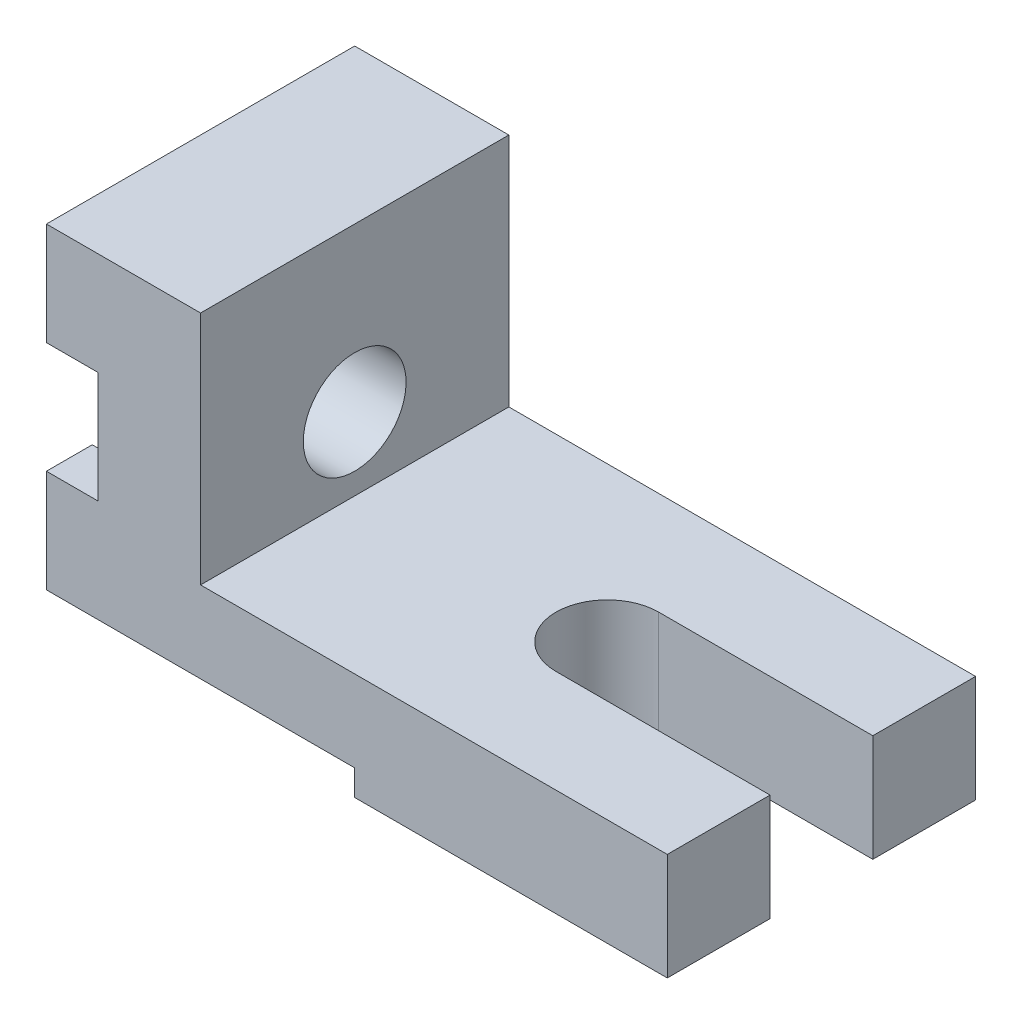
ISO-10303-21;
HEADER;
FILE_DESCRIPTION(('STEP AP214'),'2;1');
FILE_NAME('part.step','',(''),(''),'','','');
FILE_SCHEMA(('AUTOMOTIVE_DESIGN { 1 0 10303 214 1 1 1 1 }'));
ENDSEC;
DATA;
#1=APPLICATION_CONTEXT('core data for automotive mechanical design processes');
#2=APPLICATION_PROTOCOL_DEFINITION('international standard','automotive_design',2000,#1);
#3=PRODUCT_CONTEXT('',#1,'mechanical');
#4=PRODUCT('Part','Part','',(#3));
#5=PRODUCT_RELATED_PRODUCT_CATEGORY('part','',(#4));
#6=PRODUCT_DEFINITION_FORMATION('','',#4);
#7=PRODUCT_DEFINITION_CONTEXT('part definition',#1,'design');
#8=PRODUCT_DEFINITION('design','',#6,#7);
#9=PRODUCT_DEFINITION_SHAPE('','',#8);
#10=(LENGTH_UNIT() NAMED_UNIT(*) SI_UNIT(.MILLI.,.METRE.));
#11=(NAMED_UNIT(*) PLANE_ANGLE_UNIT() SI_UNIT($,.RADIAN.));
#12=(NAMED_UNIT(*) SI_UNIT($,.STERADIAN.) SOLID_ANGLE_UNIT());
#13=UNCERTAINTY_MEASURE_WITH_UNIT(LENGTH_MEASURE(1.E-05),#10,'distance_accuracy_value','');
#14=(GEOMETRIC_REPRESENTATION_CONTEXT(3) GLOBAL_UNCERTAINTY_ASSIGNED_CONTEXT((#13)) GLOBAL_UNIT_ASSIGNED_CONTEXT((#10,
#11,#12)) REPRESENTATION_CONTEXT('',''));
#15=CARTESIAN_POINT('',(0.,0.,0.));
#16=DIRECTION('',(0.,0.,1.));
#17=DIRECTION('',(1.,0.,0.));
#18=AXIS2_PLACEMENT_3D('',#15,#16,#17);
#19=CARTESIAN_POINT('',(0.,30.,0.));
#20=DIRECTION('',(0.,1.,0.));
#21=DIRECTION('',(0.,0.,1.));
#22=AXIS2_PLACEMENT_3D('',#19,#20,#21);
#23=PLANE('',#22);
#24=DIRECTION('',(-1.,0.,0.));
#25=VECTOR('',#24,1.);
#26=CARTESIAN_POINT('',(-60.5,30.,-25.298221281347));
#27=LINE('',#26,#25);
#28=CARTESIAN_POINT('',(-60.5,30.,-25.298221281347));
#29=VERTEX_POINT('',#28);
#30=CARTESIAN_POINT('',(-72.5,30.,-25.298221281347));
#31=VERTEX_POINT('',#30);
#32=EDGE_CURVE('E362',#29,#31,#27,.T.);
#33=ORIENTED_EDGE('',*,*,#32,.F.);
#34=DIRECTION('',(0.,0.,-1.));
#35=VECTOR('',#34,1.);
#36=CARTESIAN_POINT('',(-60.5,30.,-36.));
#37=LINE('',#36,#35);
#38=CARTESIAN_POINT('',(-60.5,30.,-36.));
#39=VERTEX_POINT('',#38);
#40=EDGE_CURVE('E224',#29,#39,#37,.T.);
#41=ORIENTED_EDGE('',*,*,#40,.T.);
#42=DIRECTION('',(-1.,0.,0.));
#43=VECTOR('',#42,1.);
#44=CARTESIAN_POINT('',(-72.5,30.,-36.));
#45=LINE('',#44,#43);
#46=CARTESIAN_POINT('',(-72.5,30.,-36.));
#47=VERTEX_POINT('',#46);
#48=EDGE_CURVE('E230',#39,#47,#45,.T.);
#49=ORIENTED_EDGE('',*,*,#48,.T.);
#50=DIRECTION('',(0.,0.,1.));
#51=VECTOR('',#50,1.);
#52=CARTESIAN_POINT('',(-72.5,30.,-36.));
#53=LINE('',#52,#51);
#54=EDGE_CURVE('E220',#47,#31,#53,.T.);
#55=ORIENTED_EDGE('',*,*,#54,.T.);
#56=EDGE_LOOP('',(#33,#41,#49,#55));
#57=FACE_BOUND('',#56,.T.);
#58=ADVANCED_FACE('F39',(#57),#23,.T.);
#59=CARTESIAN_POINT('',(-60.5,56.,-36.));
#60=DIRECTION('',(0.,-1.,0.));
#61=DIRECTION('',(0.,0.,-1.));
#62=AXIS2_PLACEMENT_3D('',#59,#60,#61);
#63=PLANE('',#62);
#64=DIRECTION('',(-1.,0.,0.));
#65=VECTOR('',#64,1.);
#66=CARTESIAN_POINT('',(-60.5,56.,24.2487113059643));
#67=LINE('',#66,#65);
#68=CARTESIAN_POINT('',(-60.5,56.,24.2487113059643));
#69=VERTEX_POINT('',#68);
#70=CARTESIAN_POINT('',(-72.5,56.,24.2487113059643));
#71=VERTEX_POINT('',#70);
#72=EDGE_CURVE('E61',#69,#71,#67,.T.);
#73=ORIENTED_EDGE('',*,*,#72,.F.);
#74=DIRECTION('',(0.,0.,1.));
#75=VECTOR('',#74,1.);
#76=CARTESIAN_POINT('',(-60.5,56.,-36.));
#77=LINE('',#76,#75);
#78=CARTESIAN_POINT('',(-60.5,56.,36.));
#79=VERTEX_POINT('',#78);
#80=EDGE_CURVE('E194',#69,#79,#77,.T.);
#81=ORIENTED_EDGE('',*,*,#80,.T.);
#82=DIRECTION('',(1.,0.,0.));
#83=VECTOR('',#82,1.);
#84=CARTESIAN_POINT('',(-60.5,56.,36.));
#85=LINE('',#84,#83);
#86=CARTESIAN_POINT('',(-72.5,56.,36.));
#87=VERTEX_POINT('',#86);
#88=EDGE_CURVE('E377',#87,#79,#85,.T.);
#89=ORIENTED_EDGE('',*,*,#88,.F.);
#90=DIRECTION('',(0.,0.,1.));
#91=VECTOR('',#90,1.);
#92=CARTESIAN_POINT('',(-72.5,56.,-36.));
#93=LINE('',#92,#91);
#94=EDGE_CURVE('E195',#71,#87,#93,.T.);
#95=ORIENTED_EDGE('',*,*,#94,.F.);
#96=EDGE_LOOP('',(#73,#81,#89,#95));
#97=FACE_BOUND('',#96,.T.);
#98=ADVANCED_FACE('F189',(#97),#63,.T.);
#99=CARTESIAN_POINT('',(0.,25.,0.));
#100=DIRECTION('',(0.,-1.,0.));
#101=DIRECTION('',(0.,0.,-1.));
#102=AXIS2_PLACEMENT_3D('',#99,#100,#101);
#103=PLANE('',#102);
#104=DIRECTION('',(-1.,0.,0.));
#105=VECTOR('',#104,1.);
#106=CARTESIAN_POINT('',(-72.5,25.,-36.));
#107=LINE('',#106,#105);
#108=CARTESIAN_POINT('',(72.5,25.,-36.));
#109=VERTEX_POINT('',#108);
#110=CARTESIAN_POINT('',(-36.5,25.,-36.));
#111=VERTEX_POINT('',#110);
#112=EDGE_CURVE('E273',#109,#111,#107,.T.);
#113=ORIENTED_EDGE('',*,*,#112,.T.);
#114=DIRECTION('',(0.,0.,1.));
#115=VECTOR('',#114,1.);
#116=CARTESIAN_POINT('',(-36.5,25.,-36.));
#117=LINE('',#116,#115);
#118=CARTESIAN_POINT('',(-36.5,25.,36.));
#119=VERTEX_POINT('',#118);
#120=EDGE_CURVE('E213',#111,#119,#117,.T.);
#121=ORIENTED_EDGE('',*,*,#120,.T.);
#122=DIRECTION('',(1.,0.,0.));
#123=VECTOR('',#122,1.);
#124=CARTESIAN_POINT('',(-72.5,25.,36.));
#125=LINE('',#124,#123);
#126=CARTESIAN_POINT('',(72.5,25.,36.));
#127=VERTEX_POINT('',#126);
#128=EDGE_CURVE('E279',#119,#127,#125,.T.);
#129=ORIENTED_EDGE('',*,*,#128,.T.);
#130=DIRECTION('',(0.,0.,-1.));
#131=VECTOR('',#130,1.);
#132=CARTESIAN_POINT('',(72.5,25.,36.));
#133=LINE('',#132,#131);
#134=CARTESIAN_POINT('',(72.5,25.,12.));
#135=VERTEX_POINT('',#134);
#136=EDGE_CURVE('E271',#127,#135,#133,.T.);
#137=ORIENTED_EDGE('',*,*,#136,.T.);
#138=DIRECTION('',(1.,0.,0.));
#139=VECTOR('',#138,1.);
#140=CARTESIAN_POINT('',(72.5,25.,12.));
#141=LINE('',#140,#139);
#142=CARTESIAN_POINT('',(22.5,25.,12.));
#143=VERTEX_POINT('',#142);
#144=EDGE_CURVE('E235',#143,#135,#141,.T.);
#145=ORIENTED_EDGE('',*,*,#144,.F.);
#146=CARTESIAN_POINT('',(22.5,25.,0.));
#147=DIRECTION('',(0.,1.,0.));
#148=DIRECTION('',(0.,0.,1.));
#149=AXIS2_PLACEMENT_3D('',#146,#147,#148);
#150=CIRCLE('',#149,12.);
#151=CARTESIAN_POINT('',(22.5,25.,-12.));
#152=VERTEX_POINT('',#151);
#153=EDGE_CURVE('E227',#152,#143,#150,.T.);
#154=ORIENTED_EDGE('',*,*,#153,.F.);
#155=DIRECTION('',(-1.,0.,0.));
#156=VECTOR('',#155,1.);
#157=CARTESIAN_POINT('',(22.5,25.,-12.));
#158=LINE('',#157,#156);
#159=CARTESIAN_POINT('',(72.5,25.,-12.));
#160=VERTEX_POINT('',#159);
#161=EDGE_CURVE('E232',#160,#152,#158,.T.);
#162=ORIENTED_EDGE('',*,*,#161,.F.);
#163=EDGE_CURVE('E274',#160,#109,#133,.T.);
#164=ORIENTED_EDGE('',*,*,#163,.T.);
#165=EDGE_LOOP('',(#113,#121,#129,#137,#145,#154,#162,#164));
#166=FACE_BOUND('',#165,.T.);
#167=ADVANCED_FACE('F326',(#166),#103,.F.);
#168=CARTESIAN_POINT('',(72.5,25.,36.));
#169=DIRECTION('',(-1.,0.,0.));
#170=DIRECTION('',(0.,0.,1.));
#171=AXIS2_PLACEMENT_3D('',#168,#169,#170);
#172=PLANE('',#171);
#173=ORIENTED_EDGE('',*,*,#163,.F.);
#174=DIRECTION('',(0.,1.,0.));
#175=VECTOR('',#174,1.);
#176=CARTESIAN_POINT('',(72.5,-25.,-12.));
#177=LINE('',#176,#175);
#178=CARTESIAN_POINT('',(72.5,0.,-12.));
#179=VERTEX_POINT('',#178);
#180=EDGE_CURVE('E245',#179,#160,#177,.T.);
#181=ORIENTED_EDGE('',*,*,#180,.F.);
#182=DIRECTION('',(0.,0.,-1.));
#183=VECTOR('',#182,1.);
#184=CARTESIAN_POINT('',(72.5,0.,36.));
#185=LINE('',#184,#183);
#186=CARTESIAN_POINT('',(72.5,0.,-36.));
#187=VERTEX_POINT('',#186);
#188=EDGE_CURVE('E270',#179,#187,#185,.T.);
#189=ORIENTED_EDGE('',*,*,#188,.T.);
#190=DIRECTION('',(0.,-1.,0.));
#191=VECTOR('',#190,1.);
#192=CARTESIAN_POINT('',(72.5,25.,-36.));
#193=LINE('',#192,#191);
#194=EDGE_CURVE('E299',#109,#187,#193,.T.);
#195=ORIENTED_EDGE('',*,*,#194,.F.);
#196=EDGE_LOOP('',(#173,#181,#189,#195));
#197=FACE_BOUND('',#196,.T.);
#198=ADVANCED_FACE('F322',(#197),#172,.F.);
#199=CARTESIAN_POINT('',(72.5,0.,36.));
#200=VERTEX_POINT('',#199);
#201=CARTESIAN_POINT('',(72.5,0.,12.));
#202=VERTEX_POINT('',#201);
#203=EDGE_CURVE('E283',#200,#202,#185,.T.);
#204=ORIENTED_EDGE('',*,*,#203,.T.);
#205=DIRECTION('',(0.,1.,0.));
#206=VECTOR('',#205,1.);
#207=CARTESIAN_POINT('',(72.5,-25.,12.));
#208=LINE('',#207,#206);
#209=EDGE_CURVE('E244',#202,#135,#208,.T.);
#210=ORIENTED_EDGE('',*,*,#209,.T.);
#211=ORIENTED_EDGE('',*,*,#136,.F.);
#212=DIRECTION('',(0.,-1.,0.));
#213=VECTOR('',#212,1.);
#214=CARTESIAN_POINT('',(72.5,25.,36.));
#215=LINE('',#214,#213);
#216=EDGE_CURVE('E278',#127,#200,#215,.T.);
#217=ORIENTED_EDGE('',*,*,#216,.T.);
#218=EDGE_LOOP('',(#204,#210,#211,#217));
#219=FACE_BOUND('',#218,.T.);
#220=ADVANCED_FACE('F41',(#219),#172,.F.);
#221=CARTESIAN_POINT('',(-72.5,25.,-36.));
#222=DIRECTION('',(0.,0.,1.));
#223=DIRECTION('',(1.,0.,0.));
#224=AXIS2_PLACEMENT_3D('',#221,#222,#223);
#225=PLANE('',#224);
#226=DIRECTION('',(0.,1.,0.));
#227=VECTOR('',#226,1.);
#228=CARTESIAN_POINT('',(-36.5,80.,-36.));
#229=LINE('',#228,#227);
#230=CARTESIAN_POINT('',(-36.5,80.,-36.));
#231=VERTEX_POINT('',#230);
#232=EDGE_CURVE('E379',#111,#231,#229,.T.);
#233=ORIENTED_EDGE('',*,*,#232,.F.);
#234=ORIENTED_EDGE('',*,*,#112,.F.);
#235=ORIENTED_EDGE('',*,*,#194,.T.);
#236=DIRECTION('',(-1.,0.,0.));
#237=VECTOR('',#236,1.);
#238=CARTESIAN_POINT('',(-72.5,0.,-36.));
#239=LINE('',#238,#237);
#240=CARTESIAN_POINT('',(-72.5,0.,-36.));
#241=VERTEX_POINT('',#240);
#242=EDGE_CURVE('E284',#187,#241,#239,.T.);
#243=ORIENTED_EDGE('',*,*,#242,.T.);
#244=DIRECTION('',(0.,-1.,0.));
#245=VECTOR('',#244,1.);
#246=CARTESIAN_POINT('',(-72.5,25.,-36.));
#247=LINE('',#246,#245);
#248=EDGE_CURVE('E298',#47,#241,#247,.T.);
#249=ORIENTED_EDGE('',*,*,#248,.F.);
#250=ORIENTED_EDGE('',*,*,#48,.F.);
#251=DIRECTION('',(0.,-1.,0.));
#252=VECTOR('',#251,1.);
#253=CARTESIAN_POINT('',(-60.5,25.,-36.));
#254=LINE('',#253,#252);
#255=CARTESIAN_POINT('',(-60.5,56.,-36.));
#256=VERTEX_POINT('',#255);
#257=EDGE_CURVE('E216',#256,#39,#254,.T.);
#258=ORIENTED_EDGE('',*,*,#257,.F.);
#259=DIRECTION('',(1.,0.,0.));
#260=VECTOR('',#259,1.);
#261=CARTESIAN_POINT('',(-60.5,56.,-36.));
#262=LINE('',#261,#260);
#263=CARTESIAN_POINT('',(-72.5,56.,-36.));
#264=VERTEX_POINT('',#263);
#265=EDGE_CURVE('E364',#264,#256,#262,.T.);
#266=ORIENTED_EDGE('',*,*,#265,.F.);
#267=DIRECTION('',(0.,-1.,0.));
#268=VECTOR('',#267,1.);
#269=CARTESIAN_POINT('',(-72.5,56.,-36.));
#270=LINE('',#269,#268);
#271=CARTESIAN_POINT('',(-72.5,80.,-36.));
#272=VERTEX_POINT('',#271);
#273=EDGE_CURVE('E370',#272,#264,#270,.T.);
#274=ORIENTED_EDGE('',*,*,#273,.F.);
#275=DIRECTION('',(-1.,0.,0.));
#276=VECTOR('',#275,1.);
#277=CARTESIAN_POINT('',(-72.5,80.,-36.));
#278=LINE('',#277,#276);
#279=EDGE_CURVE('E382',#231,#272,#278,.T.);
#280=ORIENTED_EDGE('',*,*,#279,.F.);
#281=EDGE_LOOP('',(#233,#234,#235,#243,#249,#250,#258,#266,#274,#280));
#282=FACE_BOUND('',#281,.T.);
#283=ADVANCED_FACE('F356',(#282),#225,.F.);
#284=CARTESIAN_POINT('',(-72.5,25.,36.));
#285=DIRECTION('',(1.,0.,0.));
#286=DIRECTION('',(0.,0.,-1.));
#287=AXIS2_PLACEMENT_3D('',#284,#285,#286);
#288=PLANE('',#287);
#289=CARTESIAN_POINT('',(-72.5,30.,25.298221281347));
#290=VERTEX_POINT('',#289);
#291=CARTESIAN_POINT('',(-72.5,30.,36.));
#292=VERTEX_POINT('',#291);
#293=EDGE_CURVE('E201',#290,#292,#53,.T.);
#294=ORIENTED_EDGE('',*,*,#293,.F.);
#295=CARTESIAN_POINT('',(-72.5,42.,0.));
#296=DIRECTION('',(-1.,0.,0.));
#297=DIRECTION('',(0.,0.,1.));
#298=AXIS2_PLACEMENT_3D('',#295,#296,#297);
#299=CIRCLE('',#298,28.);
#300=EDGE_CURVE('E402',#31,#290,#299,.T.);
#301=ORIENTED_EDGE('',*,*,#300,.F.);
#302=ORIENTED_EDGE('',*,*,#54,.F.);
#303=ORIENTED_EDGE('',*,*,#248,.T.);
#304=DIRECTION('',(0.,0.,1.));
#305=VECTOR('',#304,1.);
#306=CARTESIAN_POINT('',(-72.5,0.,36.));
#307=LINE('',#306,#305);
#308=CARTESIAN_POINT('',(-72.5,0.,-14.));
#309=VERTEX_POINT('',#308);
#310=EDGE_CURVE('E289',#241,#309,#307,.T.);
#311=ORIENTED_EDGE('',*,*,#310,.T.);
#312=DIRECTION('',(0.,-1.,0.));
#313=VECTOR('',#312,1.);
#314=CARTESIAN_POINT('',(-72.5,0.,-14.));
#315=LINE('',#314,#313);
#316=CARTESIAN_POINT('',(-72.5,6.,-14.));
#317=VERTEX_POINT('',#316);
#318=EDGE_CURVE('E250',#317,#309,#315,.T.);
#319=ORIENTED_EDGE('',*,*,#318,.F.);
#320=DIRECTION('',(0.,0.,1.));
#321=VECTOR('',#320,1.);
#322=CARTESIAN_POINT('',(-72.5,6.,-14.));
#323=LINE('',#322,#321);
#324=CARTESIAN_POINT('',(-72.5,6.,36.));
#325=VERTEX_POINT('',#324);
#326=EDGE_CURVE('E262',#317,#325,#323,.T.);
#327=ORIENTED_EDGE('',*,*,#326,.T.);
#328=DIRECTION('',(0.,-1.,0.));
#329=VECTOR('',#328,1.);
#330=CARTESIAN_POINT('',(-72.5,25.,36.));
#331=LINE('',#330,#329);
#332=EDGE_CURVE('E291',#292,#325,#331,.T.);
#333=ORIENTED_EDGE('',*,*,#332,.F.);
#334=EDGE_LOOP('',(#294,#301,#302,#303,#311,#319,#327,#333));
#335=FACE_BOUND('',#334,.T.);
#336=ADVANCED_FACE('F353',(#335),#288,.F.);
#337=CARTESIAN_POINT('',(-72.5,25.,36.));
#338=DIRECTION('',(0.,0.,-1.));
#339=DIRECTION('',(-1.,0.,0.));
#340=AXIS2_PLACEMENT_3D('',#337,#338,#339);
#341=PLANE('',#340);
#342=ORIENTED_EDGE('',*,*,#128,.F.);
#343=DIRECTION('',(0.,1.,0.));
#344=VECTOR('',#343,1.);
#345=CARTESIAN_POINT('',(-36.5,80.,36.));
#346=LINE('',#345,#344);
#347=CARTESIAN_POINT('',(-36.5,80.,36.));
#348=VERTEX_POINT('',#347);
#349=EDGE_CURVE('E371',#119,#348,#346,.T.);
#350=ORIENTED_EDGE('',*,*,#349,.T.);
#351=DIRECTION('',(-1.,0.,0.));
#352=VECTOR('',#351,1.);
#353=CARTESIAN_POINT('',(-72.5,80.,36.));
#354=LINE('',#353,#352);
#355=CARTESIAN_POINT('',(-72.5,80.,36.));
#356=VERTEX_POINT('',#355);
#357=EDGE_CURVE('E372',#348,#356,#354,.T.);
#358=ORIENTED_EDGE('',*,*,#357,.T.);
#359=DIRECTION('',(0.,-1.,0.));
#360=VECTOR('',#359,1.);
#361=CARTESIAN_POINT('',(-72.5,56.,36.));
#362=LINE('',#361,#360);
#363=EDGE_CURVE('E380',#356,#87,#362,.T.);
#364=ORIENTED_EDGE('',*,*,#363,.T.);
#365=ORIENTED_EDGE('',*,*,#88,.T.);
#366=DIRECTION('',(0.,-1.,0.));
#367=VECTOR('',#366,1.);
#368=CARTESIAN_POINT('',(-60.5,25.,36.));
#369=LINE('',#368,#367);
#370=CARTESIAN_POINT('',(-60.5,30.,36.));
#371=VERTEX_POINT('',#370);
#372=EDGE_CURVE('E200',#79,#371,#369,.T.);
#373=ORIENTED_EDGE('',*,*,#372,.T.);
#374=DIRECTION('',(1.,0.,0.));
#375=VECTOR('',#374,1.);
#376=CARTESIAN_POINT('',(-72.5,30.,36.));
#377=LINE('',#376,#375);
#378=EDGE_CURVE('E219',#292,#371,#377,.T.);
#379=ORIENTED_EDGE('',*,*,#378,.F.);
#380=ORIENTED_EDGE('',*,*,#332,.T.);
#381=DIRECTION('',(-1.,0.,0.));
#382=VECTOR('',#381,1.);
#383=CARTESIAN_POINT('',(-72.5,6.,36.));
#384=LINE('',#383,#382);
#385=CARTESIAN_POINT('',(-0.5,6.,36.));
#386=VERTEX_POINT('',#385);
#387=EDGE_CURVE('E253',#386,#325,#384,.T.);
#388=ORIENTED_EDGE('',*,*,#387,.F.);
#389=DIRECTION('',(0.,1.,0.));
#390=VECTOR('',#389,1.);
#391=CARTESIAN_POINT('',(-0.5,0.,36.));
#392=LINE('',#391,#390);
#393=CARTESIAN_POINT('',(-0.5,0.,36.));
#394=VERTEX_POINT('',#393);
#395=EDGE_CURVE('E243',#394,#386,#392,.T.);
#396=ORIENTED_EDGE('',*,*,#395,.F.);
#397=DIRECTION('',(1.,0.,0.));
#398=VECTOR('',#397,1.);
#399=CARTESIAN_POINT('',(-72.5,0.,36.));
#400=LINE('',#399,#398);
#401=EDGE_CURVE('E288',#394,#200,#400,.T.);
#402=ORIENTED_EDGE('',*,*,#401,.T.);
#403=ORIENTED_EDGE('',*,*,#216,.F.);
#404=EDGE_LOOP('',(#342,#350,#358,#364,#365,#373,#379,#380,#388,#396,#402,#403));
#405=FACE_BOUND('',#404,.T.);
#406=ADVANCED_FACE('F344',(#405),#341,.F.);
#407=CARTESIAN_POINT('',(0.,0.,0.));
#408=DIRECTION('',(0.,-1.,0.));
#409=DIRECTION('',(0.,0.,-1.));
#410=AXIS2_PLACEMENT_3D('',#407,#408,#409);
#411=PLANE('',#410);
#412=DIRECTION('',(1.,0.,0.));
#413=VECTOR('',#412,1.);
#414=CARTESIAN_POINT('',(0.,0.,-12.));
#415=LINE('',#414,#413);
#416=CARTESIAN_POINT('',(22.5,0.,-12.));
#417=VERTEX_POINT('',#416);
#418=EDGE_CURVE('E11',#417,#179,#415,.T.);
#419=ORIENTED_EDGE('',*,*,#418,.F.);
#420=CARTESIAN_POINT('',(22.5,0.,0.));
#421=DIRECTION('',(0.,-1.,0.));
#422=DIRECTION('',(0.,0.,-1.));
#423=AXIS2_PLACEMENT_3D('',#420,#421,#422);
#424=CIRCLE('',#423,12.);
#425=CARTESIAN_POINT('',(22.5,0.,12.));
#426=VERTEX_POINT('',#425);
#427=EDGE_CURVE('E48',#426,#417,#424,.T.);
#428=ORIENTED_EDGE('',*,*,#427,.F.);
#429=DIRECTION('',(-1.,0.,0.));
#430=VECTOR('',#429,1.);
#431=CARTESIAN_POINT('',(0.,0.,12.));
#432=LINE('',#431,#430);
#433=EDGE_CURVE('E301',#202,#426,#432,.T.);
#434=ORIENTED_EDGE('',*,*,#433,.F.);
#435=ORIENTED_EDGE('',*,*,#203,.F.);
#436=ORIENTED_EDGE('',*,*,#401,.F.);
#437=DIRECTION('',(0.,0.,1.));
#438=VECTOR('',#437,1.);
#439=CARTESIAN_POINT('',(-0.5,0.,-14.));
#440=LINE('',#439,#438);
#441=CARTESIAN_POINT('',(-0.5,0.,-14.));
#442=VERTEX_POINT('',#441);
#443=EDGE_CURVE('E257',#442,#394,#440,.T.);
#444=ORIENTED_EDGE('',*,*,#443,.F.);
#445=DIRECTION('',(1.,0.,0.));
#446=VECTOR('',#445,1.);
#447=CARTESIAN_POINT('',(-72.5,0.,-14.));
#448=LINE('',#447,#446);
#449=EDGE_CURVE('E247',#309,#442,#448,.T.);
#450=ORIENTED_EDGE('',*,*,#449,.F.);
#451=ORIENTED_EDGE('',*,*,#310,.F.);
#452=ORIENTED_EDGE('',*,*,#242,.F.);
#453=ORIENTED_EDGE('',*,*,#188,.F.);
#454=EDGE_LOOP('',(#419,#428,#434,#435,#436,#444,#450,#451,#452,#453));
#455=FACE_BOUND('',#454,.T.);
#456=ADVANCED_FACE('F318',(#455),#411,.T.);
#457=CARTESIAN_POINT('',(-72.5,6.,-14.));
#458=DIRECTION('',(0.,1.,0.));
#459=DIRECTION('',(0.,0.,1.));
#460=AXIS2_PLACEMENT_3D('',#457,#458,#459);
#461=PLANE('',#460);
#462=ORIENTED_EDGE('',*,*,#387,.T.);
#463=ORIENTED_EDGE('',*,*,#326,.F.);
#464=DIRECTION('',(-1.,0.,0.));
#465=VECTOR('',#464,1.);
#466=CARTESIAN_POINT('',(-72.5,6.,-14.));
#467=LINE('',#466,#465);
#468=CARTESIAN_POINT('',(-0.5,6.,-14.));
#469=VERTEX_POINT('',#468);
#470=EDGE_CURVE('E260',#469,#317,#467,.T.);
#471=ORIENTED_EDGE('',*,*,#470,.F.);
#472=DIRECTION('',(0.,0.,1.));
#473=VECTOR('',#472,1.);
#474=CARTESIAN_POINT('',(-0.5,6.,-14.));
#475=LINE('',#474,#473);
#476=EDGE_CURVE('E268',#469,#386,#475,.T.);
#477=ORIENTED_EDGE('',*,*,#476,.T.);
#478=EDGE_LOOP('',(#462,#463,#471,#477));
#479=FACE_BOUND('',#478,.T.);
#480=ADVANCED_FACE('F562',(#479),#461,.F.);
#481=CARTESIAN_POINT('',(-0.5,0.,-14.));
#482=DIRECTION('',(1.,0.,0.));
#483=DIRECTION('',(0.,0.,-1.));
#484=AXIS2_PLACEMENT_3D('',#481,#482,#483);
#485=PLANE('',#484);
#486=ORIENTED_EDGE('',*,*,#395,.T.);
#487=ORIENTED_EDGE('',*,*,#476,.F.);
#488=DIRECTION('',(0.,1.,0.));
#489=VECTOR('',#488,1.);
#490=CARTESIAN_POINT('',(-0.5,0.,-14.));
#491=LINE('',#490,#489);
#492=EDGE_CURVE('E255',#442,#469,#491,.T.);
#493=ORIENTED_EDGE('',*,*,#492,.F.);
#494=ORIENTED_EDGE('',*,*,#443,.T.);
#495=EDGE_LOOP('',(#486,#487,#493,#494));
#496=FACE_BOUND('',#495,.T.);
#497=ADVANCED_FACE('F343',(#496),#485,.F.);
#498=CARTESIAN_POINT('',(0.,0.,-14.));
#499=DIRECTION('',(0.,0.,-1.));
#500=DIRECTION('',(-1.,0.,0.));
#501=AXIS2_PLACEMENT_3D('',#498,#499,#500);
#502=PLANE('',#501);
#503=ORIENTED_EDGE('',*,*,#318,.T.);
#504=ORIENTED_EDGE('',*,*,#449,.T.);
#505=ORIENTED_EDGE('',*,*,#492,.T.);
#506=ORIENTED_EDGE('',*,*,#470,.T.);
#507=EDGE_LOOP('',(#503,#504,#505,#506));
#508=FACE_BOUND('',#507,.T.);
#509=ADVANCED_FACE('F350',(#508),#502,.F.);
#510=CARTESIAN_POINT('',(22.5,-25.,0.));
#511=DIRECTION('',(0.,1.,0.));
#512=DIRECTION('',(0.,0.,1.));
#513=AXIS2_PLACEMENT_3D('',#510,#511,#512);
#514=CYLINDRICAL_SURFACE('',#513,12.);
#515=ORIENTED_EDGE('',*,*,#427,.T.);
#516=DIRECTION('',(0.,1.,0.));
#517=VECTOR('',#516,1.);
#518=CARTESIAN_POINT('',(22.5,-25.,-12.));
#519=LINE('',#518,#517);
#520=EDGE_CURVE('E239',#417,#152,#519,.T.);
#521=ORIENTED_EDGE('',*,*,#520,.T.);
#522=ORIENTED_EDGE('',*,*,#153,.T.);
#523=DIRECTION('',(0.,1.,0.));
#524=VECTOR('',#523,1.);
#525=CARTESIAN_POINT('',(22.5,-25.,12.));
#526=LINE('',#525,#524);
#527=EDGE_CURVE('E236',#426,#143,#526,.T.);
#528=ORIENTED_EDGE('',*,*,#527,.F.);
#529=EDGE_LOOP('',(#515,#521,#522,#528));
#530=FACE_BOUND('',#529,.T.);
#531=ADVANCED_FACE('F306',(#530),#514,.F.);
#532=CARTESIAN_POINT('',(22.5,-25.,-12.));
#533=DIRECTION('',(0.,0.,-1.));
#534=DIRECTION('',(-1.,0.,0.));
#535=AXIS2_PLACEMENT_3D('',#532,#533,#534);
#536=PLANE('',#535);
#537=ORIENTED_EDGE('',*,*,#418,.T.);
#538=ORIENTED_EDGE('',*,*,#180,.T.);
#539=ORIENTED_EDGE('',*,*,#161,.T.);
#540=ORIENTED_EDGE('',*,*,#520,.F.);
#541=EDGE_LOOP('',(#537,#538,#539,#540));
#542=FACE_BOUND('',#541,.T.);
#543=ADVANCED_FACE('F311',(#542),#536,.F.);
#544=CARTESIAN_POINT('',(72.5,-25.,12.));
#545=DIRECTION('',(0.,0.,1.));
#546=DIRECTION('',(1.,0.,0.));
#547=AXIS2_PLACEMENT_3D('',#544,#545,#546);
#548=PLANE('',#547);
#549=ORIENTED_EDGE('',*,*,#433,.T.);
#550=ORIENTED_EDGE('',*,*,#527,.T.);
#551=ORIENTED_EDGE('',*,*,#144,.T.);
#552=ORIENTED_EDGE('',*,*,#209,.F.);
#553=EDGE_LOOP('',(#549,#550,#551,#552));
#554=FACE_BOUND('',#553,.T.);
#555=ADVANCED_FACE('F332',(#554),#548,.F.);
#556=DIRECTION('',(-1.,0.,0.));
#557=VECTOR('',#556,1.);
#558=CARTESIAN_POINT('',(-60.5,30.,25.298221281347));
#559=LINE('',#558,#557);
#560=CARTESIAN_POINT('',(-60.5,30.,25.298221281347));
#561=VERTEX_POINT('',#560);
#562=EDGE_CURVE('E193',#290,#561,#559,.F.);
#563=ORIENTED_EDGE('',*,*,#562,.F.);
#564=ORIENTED_EDGE('',*,*,#293,.T.);
#565=ORIENTED_EDGE('',*,*,#378,.T.);
#566=EDGE_CURVE('E221',#371,#561,#37,.T.);
#567=ORIENTED_EDGE('',*,*,#566,.T.);
#568=EDGE_LOOP('',(#563,#564,#565,#567));
#569=FACE_BOUND('',#568,.T.);
#570=ADVANCED_FACE('F407',(#569),#23,.T.);
#571=CARTESIAN_POINT('',(-60.5,25.,-36.));
#572=DIRECTION('',(-1.,0.,0.));
#573=DIRECTION('',(0.,0.,1.));
#574=AXIS2_PLACEMENT_3D('',#571,#572,#573);
#575=PLANE('',#574);
#576=CARTESIAN_POINT('',(-60.5,42.,0.));
#577=DIRECTION('',(-1.,0.,0.));
#578=DIRECTION('',(0.,0.,1.));
#579=AXIS2_PLACEMENT_3D('',#576,#577,#578);
#580=CIRCLE('',#579,12.);
#581=CARTESIAN_POINT('',(-60.5,42.,12.));
#582=VERTEX_POINT('',#581);
#583=EDGE_CURVE('E455',#582,#582,#580,.T.);
#584=ORIENTED_EDGE('',*,*,#583,.F.);
#585=EDGE_LOOP('',(#584));
#586=FACE_BOUND('',#585,.T.);
#587=ORIENTED_EDGE('',*,*,#80,.F.);
#588=CARTESIAN_POINT('',(-60.5,42.,0.));
#589=DIRECTION('',(-1.,0.,0.));
#590=DIRECTION('',(0.,0.,1.));
#591=AXIS2_PLACEMENT_3D('',#588,#589,#590);
#592=CIRCLE('',#591,28.);
#593=CARTESIAN_POINT('',(-60.5,56.,-24.2487113059643));
#594=VERTEX_POINT('',#593);
#595=EDGE_CURVE('E177',#69,#594,#592,.T.);
#596=ORIENTED_EDGE('',*,*,#595,.T.);
#597=EDGE_CURVE('E199',#256,#594,#77,.T.);
#598=ORIENTED_EDGE('',*,*,#597,.F.);
#599=ORIENTED_EDGE('',*,*,#257,.T.);
#600=ORIENTED_EDGE('',*,*,#40,.F.);
#601=EDGE_CURVE('E54',#29,#561,#592,.T.);
#602=ORIENTED_EDGE('',*,*,#601,.T.);
#603=ORIENTED_EDGE('',*,*,#566,.F.);
#604=ORIENTED_EDGE('',*,*,#372,.F.);
#605=EDGE_LOOP('',(#587,#596,#598,#599,#600,#602,#603,#604));
#606=FACE_BOUND('',#605,.T.);
#607=ADVANCED_FACE('F197',(#586,#606),#575,.T.);
#608=DIRECTION('',(-1.,0.,0.));
#609=VECTOR('',#608,1.);
#610=CARTESIAN_POINT('',(-60.5,56.,-24.2487113059643));
#611=LINE('',#610,#609);
#612=CARTESIAN_POINT('',(-72.5,56.,-24.2487113059643));
#613=VERTEX_POINT('',#612);
#614=EDGE_CURVE('E181',#613,#594,#611,.F.);
#615=ORIENTED_EDGE('',*,*,#614,.F.);
#616=EDGE_CURVE('E203',#264,#613,#93,.T.);
#617=ORIENTED_EDGE('',*,*,#616,.F.);
#618=ORIENTED_EDGE('',*,*,#265,.T.);
#619=ORIENTED_EDGE('',*,*,#597,.T.);
#620=EDGE_LOOP('',(#615,#617,#618,#619));
#621=FACE_BOUND('',#620,.T.);
#622=ADVANCED_FACE('F416',(#621),#63,.T.);
#623=CARTESIAN_POINT('',(-72.5,56.,-36.));
#624=DIRECTION('',(-1.,0.,0.));
#625=DIRECTION('',(0.,0.,1.));
#626=AXIS2_PLACEMENT_3D('',#623,#624,#625);
#627=PLANE('',#626);
#628=EDGE_CURVE('E397',#71,#613,#299,.T.);
#629=ORIENTED_EDGE('',*,*,#628,.F.);
#630=ORIENTED_EDGE('',*,*,#94,.T.);
#631=ORIENTED_EDGE('',*,*,#363,.F.);
#632=DIRECTION('',(0.,0.,1.));
#633=VECTOR('',#632,1.);
#634=CARTESIAN_POINT('',(-72.5,80.,-36.));
#635=LINE('',#634,#633);
#636=EDGE_CURVE('E207',#272,#356,#635,.T.);
#637=ORIENTED_EDGE('',*,*,#636,.F.);
#638=ORIENTED_EDGE('',*,*,#273,.T.);
#639=ORIENTED_EDGE('',*,*,#616,.T.);
#640=EDGE_LOOP('',(#629,#630,#631,#637,#638,#639));
#641=FACE_BOUND('',#640,.T.);
#642=ADVANCED_FACE('F391',(#641),#627,.T.);
#643=CARTESIAN_POINT('',(-72.5,80.,-36.));
#644=DIRECTION('',(0.,1.,0.));
#645=DIRECTION('',(0.,0.,1.));
#646=AXIS2_PLACEMENT_3D('',#643,#644,#645);
#647=PLANE('',#646);
#648=ORIENTED_EDGE('',*,*,#357,.F.);
#649=DIRECTION('',(0.,0.,1.));
#650=VECTOR('',#649,1.);
#651=CARTESIAN_POINT('',(-36.5,80.,-36.));
#652=LINE('',#651,#650);
#653=EDGE_CURVE('E211',#231,#348,#652,.T.);
#654=ORIENTED_EDGE('',*,*,#653,.F.);
#655=ORIENTED_EDGE('',*,*,#279,.T.);
#656=ORIENTED_EDGE('',*,*,#636,.T.);
#657=EDGE_LOOP('',(#648,#654,#655,#656));
#658=FACE_BOUND('',#657,.T.);
#659=ADVANCED_FACE('F400',(#658),#647,.T.);
#660=CARTESIAN_POINT('',(-36.5,80.,-36.));
#661=DIRECTION('',(1.,0.,0.));
#662=DIRECTION('',(0.,1.,0.));
#663=AXIS2_PLACEMENT_3D('',#660,#661,#662);
#664=PLANE('',#663);
#665=CARTESIAN_POINT('',(-36.5,42.,0.));
#666=DIRECTION('',(1.,0.,0.));
#667=DIRECTION('',(0.,1.,0.));
#668=AXIS2_PLACEMENT_3D('',#665,#666,#667);
#669=CIRCLE('',#668,12.);
#670=CARTESIAN_POINT('',(-36.5,54.,0.));
#671=VERTEX_POINT('',#670);
#672=EDGE_CURVE('E43',#671,#671,#669,.T.);
#673=ORIENTED_EDGE('',*,*,#672,.F.);
#674=EDGE_LOOP('',(#673));
#675=FACE_BOUND('',#674,.T.);
#676=ORIENTED_EDGE('',*,*,#349,.F.);
#677=ORIENTED_EDGE('',*,*,#120,.F.);
#678=ORIENTED_EDGE('',*,*,#232,.T.);
#679=ORIENTED_EDGE('',*,*,#653,.T.);
#680=EDGE_LOOP('',(#676,#677,#678,#679));
#681=FACE_BOUND('',#680,.T.);
#682=ADVANCED_FACE('F398',(#675,#681),#664,.T.);
#683=CARTESIAN_POINT('',(-60.5,42.,0.));
#684=DIRECTION('',(-1.,0.,0.));
#685=DIRECTION('',(0.,0.,1.));
#686=AXIS2_PLACEMENT_3D('',#683,#684,#685);
#687=CYLINDRICAL_SURFACE('',#686,28.);
#688=ORIENTED_EDGE('',*,*,#72,.T.);
#689=ORIENTED_EDGE('',*,*,#628,.T.);
#690=ORIENTED_EDGE('',*,*,#614,.T.);
#691=ORIENTED_EDGE('',*,*,#595,.F.);
#692=EDGE_LOOP('',(#688,#689,#690,#691));
#693=FACE_BOUND('',#692,.T.);
#694=ADVANCED_FACE('F182',(#693),#687,.F.);
#695=ORIENTED_EDGE('',*,*,#32,.T.);
#696=ORIENTED_EDGE('',*,*,#300,.T.);
#697=ORIENTED_EDGE('',*,*,#562,.T.);
#698=ORIENTED_EDGE('',*,*,#601,.F.);
#699=EDGE_LOOP('',(#695,#696,#697,#698));
#700=FACE_BOUND('',#699,.T.);
#701=ADVANCED_FACE('F410',(#700),#687,.F.);
#702=CARTESIAN_POINT('',(72.5,42.,0.));
#703=DIRECTION('',(-1.,0.,0.));
#704=DIRECTION('',(0.,0.,1.));
#705=AXIS2_PLACEMENT_3D('',#702,#703,#704);
#706=CYLINDRICAL_SURFACE('',#705,12.);
#707=ORIENTED_EDGE('',*,*,#672,.T.);
#708=EDGE_LOOP('',(#707));
#709=FACE_BOUND('',#708,.T.);
#710=ORIENTED_EDGE('',*,*,#583,.T.);
#711=EDGE_LOOP('',(#710));
#712=FACE_BOUND('',#711,.T.);
#713=ADVANCED_FACE('F460',(#709,#712),#706,.F.);
#714=CLOSED_SHELL('',(#58,#98,#167,#198,#220,#283,#336,#406,#456,#480,#497,#509,#531,#543,#555,
#570,#607,#622,#642,#659,#682,#694,#701,#713));
#715=MANIFOLD_SOLID_BREP('B2',#714);
#716=ADVANCED_BREP_SHAPE_REPRESENTATION('',(#18,#715),#14);
#717=SHAPE_DEFINITION_REPRESENTATION(#9,#716);
ENDSEC;
END-ISO-10303-21;
